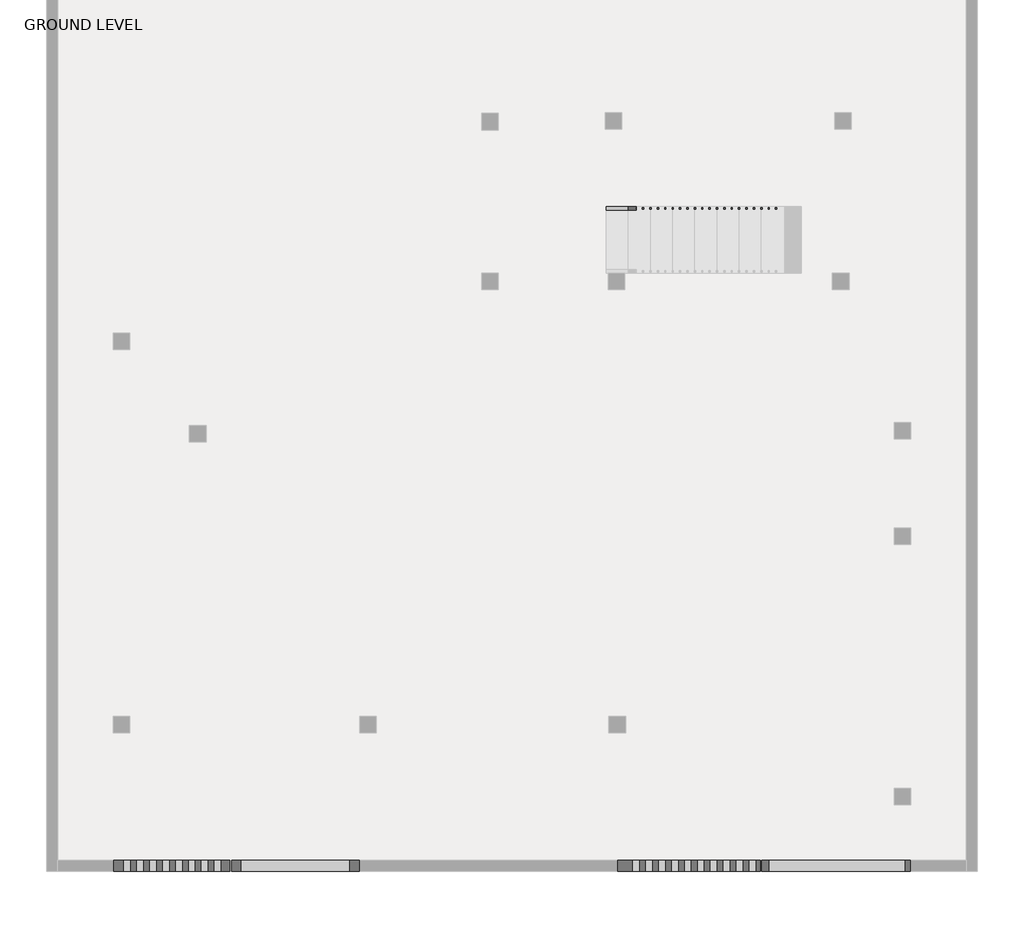
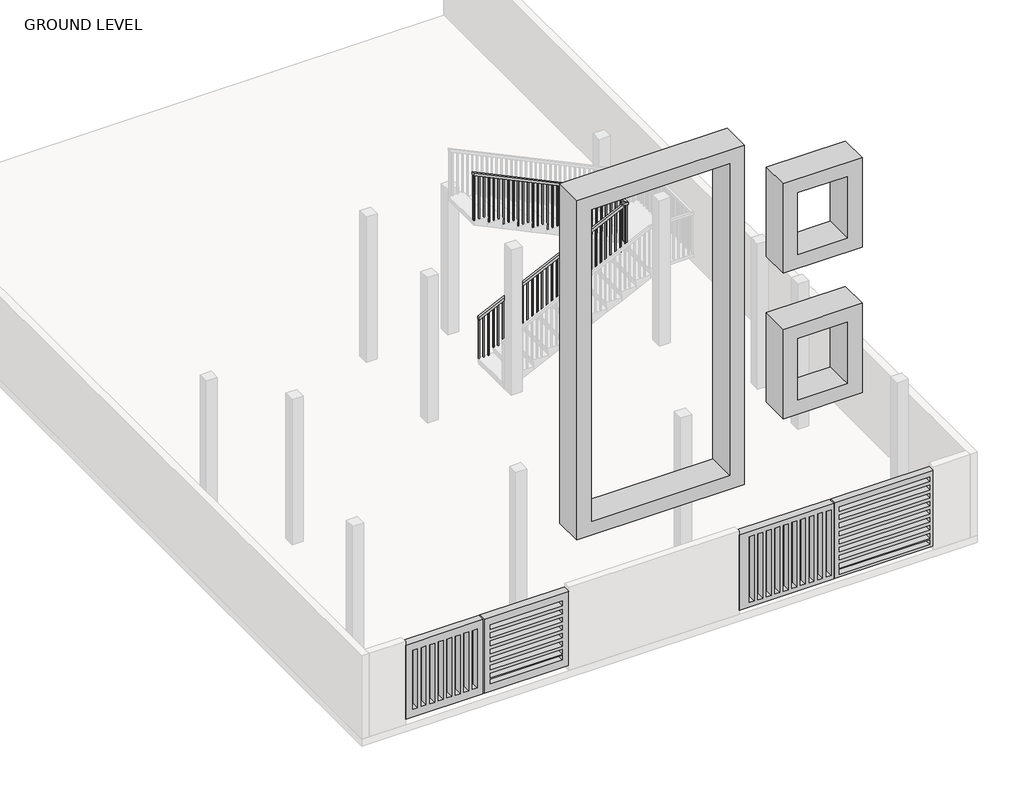
# One storey, part 3 of 3: 1 proxy, 1 railing.
"""IFC4 building model written with IfcOpenShell, lengths in millimetres."""

from ifc_helpers import new_model, si_unit, frame, origin, place, context, project, spatial, polyline, outline, extrude, faceted_brep, transform, mapped, element, save
from components import generic_models_1_generic_models_1_6b654720

model = new_model("IFC4")

# Units and contexts
model_context = context("Model", 3, world=origin())
ifc_project = project(units=[si_unit("LENGTHUNIT", "METRE", prefix="MILLI")], contexts=[model_context])

# Site, building, storey
site = spatial("IfcSite", under=ifc_project)
building = spatial("IfcBuilding", under=site)
storey = spatial("IfcBuildingStorey", under=building, Name="GROUND LEVEL", Elevation=0.0)

# Proxy
placement = place(None, origin())
generic_models_1_generic_models_1_shape = generic_models_1_generic_models_1_6b654720(model_context)
element("IfcBuildingElementProxy", 1, Name="Generic Models 1 : Generic Models 1", ObjectType="Generic Models 1 : Generic Models 1", at=placement, inside=storey, context=model_context, shape_type="MappedRepresentation", body=[
    mapped(generic_models_1_generic_models_1_shape, transform((0.0, 0.0, 0.0), x_axis=(1.0, 0.0, 0.0), y_axis=(0.0, 1.0, 0.0), z_axis=(0.0, 0.0, 1.0))),
])

# Railing
element("IfcRailing", 2, ObjectType="Handrail - Rectangular", at=placement, inside=storey, context=model_context, shape_type="SolidModel", body=[
    faceted_brep([(13.3134019, 410.1787587, 1059.8727273), (13.3134019, 410.1787587, 1003.5834559), (13.3134019, 359.3787587, 1003.5834559), (13.3134019, 359.3787587, 1059.8727273), (2985.1134019, 410.1787587, 2478.2318182), (3035.9134019, 410.1787587, 2446.1880014), (3035.9134019, 359.3787587, 2446.1880014), (2985.1134019, 359.3787587, 2478.2318182), (2985.1134019, 410.1787587, 2514.6), (3035.9134019, 410.1787587, 2463.8), (3035.9134019, 359.3787587, 2463.8), (2985.1134019, 359.3787587, 2514.6), (3061.3134019, 410.1787587, 2514.6), (3061.3134019, 410.1787587, 2463.8), (3112.1134019, 359.3787587, 2463.8), (3112.1134019, 359.3787587, 2514.6), (3061.3134019, 486.3787587, 2514.6), (3061.3134019, 537.1787587, 2463.8), (3112.1134019, 537.1787587, 2463.8), (3112.1134019, 486.3787587, 2514.6), (3061.3134019, 486.3787587, 2696.4409091), (3061.3134019, 537.1787587, 2645.6409091), (3112.1134019, 537.1787587, 2645.6409091), (3112.1134019, 486.3787587, 2696.4409091), (3061.3134019, 562.5787587, 2696.4409091), (3061.3134019, 562.5787587, 2645.6409091), (3112.1134019, 613.3787587, 2645.6409091), (3112.1134019, 613.3787587, 2696.4409091), (2985.1134019, 562.5787587, 2696.4409091), (2973.6120715, 562.5787587, 2645.6409091), (2973.6120715, 613.3787587, 2645.6409091), (2985.1134019, 613.3787587, 2696.4409091), (13.3134019, 562.5787587, 4114.8), (13.3134019, 613.3787587, 4114.8), (13.3134019, 613.3787587, 4058.5107287), (13.3134019, 562.5787587, 4058.5107287)], [[[0, 1, 2, 3]], [[1, 0, 4, 5]], [[2, 1, 5, 6]], [[3, 2, 6, 7]], [[0, 3, 7, 4]], [[5, 4, 8, 9]], [[6, 5, 9, 10]], [[7, 6, 10, 11]], [[4, 7, 11, 8]], [[9, 8, 12, 13]], [[10, 9, 13, 14]], [[11, 10, 14, 15]], [[8, 11, 15, 12]], [[13, 12, 16, 17]], [[14, 13, 17, 18]], [[15, 14, 18, 19]], [[12, 15, 19, 16]], [[17, 16, 20, 21]], [[18, 17, 21, 22]], [[19, 18, 22, 23]], [[16, 19, 23, 20]], [[21, 20, 24, 25]], [[22, 21, 25, 26]], [[23, 22, 26, 27]], [[20, 23, 27, 24]], [[25, 24, 28, 29]], [[26, 25, 29, 30]], [[27, 26, 30, 31]], [[24, 27, 31, 28]], [[32, 33, 34, 35]], [[29, 28, 32, 35]], [[30, 29, 35, 34]], [[31, 30, 34, 33]], [[28, 31, 33, 32]]]),
    extrude(outline(polyline([(4050.9340241, 29.1884019), (3054.9272727, 29.1884019), (3054.9272727, 48.2384019), (4041.8419787, 48.2384019), (4050.9340241, 29.1884019)])), frame((0.0, 578.4537587, 0.0), z_axis=(0.0, 1.0, 0.0), x_axis=(0.0, 0.0, 1.0)), (0.0, 0.0, 1.0), 19.05),
    extrude(outline(polyline([(4002.443115, 130.7884019), (3054.9272727, 130.7884019), (3054.9272727, 149.8384019), (3993.3510696, 149.8384019), (4002.443115, 130.7884019)])), frame((0.0, 578.4537587, 0.0), z_axis=(0.0, 1.0, 0.0), x_axis=(0.0, 0.0, 1.0)), (0.0, 0.0, 1.0), 19.05),
    extrude(outline(polyline([(3953.9522059, 232.3884019), (3054.9272727, 232.3884019), (3054.9272727, 251.4384019), (3944.8601605, 251.4384019), (3953.9522059, 232.3884019)])), frame((0.0, 578.4537587, 0.0), z_axis=(0.0, 1.0, 0.0), x_axis=(0.0, 0.0, 1.0)), (0.0, 0.0, 1.0), 19.05),
    extrude(outline(polyline([(3905.4612969, 333.9884019), (2909.4545455, 333.9884019), (2909.4545455, 353.0384019), (3896.3692514, 353.0384019), (3905.4612969, 333.9884019)])), frame((0.0, 578.4537587, 0.0), z_axis=(0.0, 1.0, 0.0), x_axis=(0.0, 0.0, 1.0)), (0.0, 0.0, 1.0), 19.05),
    extrude(outline(polyline([(3856.9703878, 435.5884019), (2909.4545455, 435.5884019), (2909.4545455, 454.6384019), (3847.8783423, 454.6384019), (3856.9703878, 435.5884019)])), frame((0.0, 578.4537587, 0.0), z_axis=(0.0, 1.0, 0.0), x_axis=(0.0, 0.0, 1.0)), (0.0, 0.0, 1.0), 19.05),
    extrude(outline(polyline([(3808.4794787, 537.1884019), (2909.4545455, 537.1884019), (2909.4545455, 556.2384019), (3799.3874332, 556.2384019), (3808.4794787, 537.1884019)])), frame((0.0, 578.4537587, 0.0), z_axis=(0.0, 1.0, 0.0), x_axis=(0.0, 0.0, 1.0)), (0.0, 0.0, 1.0), 19.05),
    extrude(outline(polyline([(3759.9885696, 638.7884019), (2763.9818182, 638.7884019), (2763.9818182, 657.8384019), (3750.8965241, 657.8384019), (3759.9885696, 638.7884019)])), frame((0.0, 578.4537587, 0.0), z_axis=(0.0, 1.0, 0.0), x_axis=(0.0, 0.0, 1.0)), (0.0, 0.0, 1.0), 19.05),
    extrude(outline(polyline([(3711.4976605, 740.3884019), (2763.9818182, 740.3884019), (2763.9818182, 759.4384019), (3702.405615, 759.4384019), (3711.4976605, 740.3884019)])), frame((0.0, 578.4537587, 0.0), z_axis=(0.0, 1.0, 0.0), x_axis=(0.0, 0.0, 1.0)), (0.0, 0.0, 1.0), 19.05),
    extrude(outline(polyline([(3663.0067514, 841.9884019), (2763.9818182, 841.9884019), (2763.9818182, 861.0384019), (3653.9147059, 861.0384019), (3663.0067514, 841.9884019)])), frame((0.0, 578.4537587, 0.0), z_axis=(0.0, 1.0, 0.0), x_axis=(0.0, 0.0, 1.0)), (0.0, 0.0, 1.0), 19.05),
    extrude(outline(polyline([(3614.5158423, 943.5884019), (2618.5090909, 943.5884019), (2618.5090909, 962.6384019), (3605.4237969, 962.6384019), (3614.5158423, 943.5884019)])), frame((0.0, 578.4537587, 0.0), z_axis=(0.0, 1.0, 0.0), x_axis=(0.0, 0.0, 1.0)), (0.0, 0.0, 1.0), 19.05),
    extrude(outline(polyline([(3566.0249332, 1045.1884019), (2618.5090909, 1045.1884019), (2618.5090909, 1064.2384019), (3556.9328878, 1064.2384019), (3566.0249332, 1045.1884019)])), frame((0.0, 578.4537587, 0.0), z_axis=(0.0, 1.0, 0.0), x_axis=(0.0, 0.0, 1.0)), (0.0, 0.0, 1.0), 19.05),
    extrude(outline(polyline([(3517.5340241, 1146.7884019), (2618.5090909, 1146.7884019), (2618.5090909, 1165.8384019), (3508.4419787, 1165.8384019), (3517.5340241, 1146.7884019)])), frame((0.0, 578.4537587, 0.0), z_axis=(0.0, 1.0, 0.0), x_axis=(0.0, 0.0, 1.0)), (0.0, 0.0, 1.0), 19.05),
    extrude(outline(polyline([(3469.043115, 1248.3884019), (2473.0363636, 1248.3884019), (2473.0363636, 1267.4384019), (3459.9510696, 1267.4384019), (3469.043115, 1248.3884019)])), frame((0.0, 578.4537587, 0.0), z_axis=(0.0, 1.0, 0.0), x_axis=(0.0, 0.0, 1.0)), (0.0, 0.0, 1.0), 19.05),
    extrude(outline(polyline([(3420.5522059, 1349.9884019), (2473.0363636, 1349.9884019), (2473.0363636, 1369.0384019), (3411.4601605, 1369.0384019), (3420.5522059, 1349.9884019)])), frame((0.0, 578.4537587, 0.0), z_axis=(0.0, 1.0, 0.0), x_axis=(0.0, 0.0, 1.0)), (0.0, 0.0, 1.0), 19.05),
    extrude(outline(polyline([(3372.0612969, 1451.5884019), (2473.0363636, 1451.5884019), (2473.0363636, 1470.6384019), (3362.9692514, 1470.6384019), (3372.0612969, 1451.5884019)])), frame((0.0, 578.4537587, 0.0), z_axis=(0.0, 1.0, 0.0), x_axis=(0.0, 0.0, 1.0)), (0.0, 0.0, 1.0), 19.05),
    extrude(outline(polyline([(3323.5703878, 1553.1884019), (2327.5636364, 1553.1884019), (2327.5636364, 1572.2384019), (3314.4783423, 1572.2384019), (3323.5703878, 1553.1884019)])), frame((0.0, 578.4537587, 0.0), z_axis=(0.0, 1.0, 0.0), x_axis=(0.0, 0.0, 1.0)), (0.0, 0.0, 1.0), 19.05),
    extrude(outline(polyline([(3275.0794787, 1654.7884019), (2327.5636364, 1654.7884019), (2327.5636364, 1673.8384019), (3265.9874332, 1673.8384019), (3275.0794787, 1654.7884019)])), frame((0.0, 578.4537587, 0.0), z_axis=(0.0, 1.0, 0.0), x_axis=(0.0, 0.0, 1.0)), (0.0, 0.0, 1.0), 19.05),
    extrude(outline(polyline([(3226.5885696, 1756.3884019), (2327.5636364, 1756.3884019), (2327.5636364, 1775.4384019), (3217.4965241, 1775.4384019), (3226.5885696, 1756.3884019)])), frame((0.0, 578.4537587, 0.0), z_axis=(0.0, 1.0, 0.0), x_axis=(0.0, 0.0, 1.0)), (0.0, 0.0, 1.0), 19.05),
    extrude(outline(polyline([(3178.0976605, 1857.9884019), (2182.0909091, 1857.9884019), (2182.0909091, 1877.0384019), (3169.005615, 1877.0384019), (3178.0976605, 1857.9884019)])), frame((0.0, 578.4537587, 0.0), z_axis=(0.0, 1.0, 0.0), x_axis=(0.0, 0.0, 1.0)), (0.0, 0.0, 1.0), 19.05),
    extrude(outline(polyline([(3129.6067514, 1959.5884019), (2182.0909091, 1959.5884019), (2182.0909091, 1978.6384019), (3120.5147059, 1978.6384019), (3129.6067514, 1959.5884019)])), frame((0.0, 578.4537587, 0.0), z_axis=(0.0, 1.0, 0.0), x_axis=(0.0, 0.0, 1.0)), (0.0, 0.0, 1.0), 19.05),
    extrude(outline(polyline([(3081.1158423, 2061.1884019), (2182.0909091, 2061.1884019), (2182.0909091, 2080.2384019), (3072.0237969, 2080.2384019), (3081.1158423, 2061.1884019)])), frame((0.0, 578.4537587, 0.0), z_axis=(0.0, 1.0, 0.0), x_axis=(0.0, 0.0, 1.0)), (0.0, 0.0, 1.0), 19.05),
    extrude(outline(polyline([(3032.6249332, 2162.7884019), (2036.6181818, 2162.7884019), (2036.6181818, 2181.8384019), (3023.5328878, 2181.8384019), (3032.6249332, 2162.7884019)])), frame((0.0, 578.4537587, 0.0), z_axis=(0.0, 1.0, 0.0), x_axis=(0.0, 0.0, 1.0)), (0.0, 0.0, 1.0), 19.05),
    extrude(outline(polyline([(2984.1340241, 2264.3884019), (2036.6181818, 2264.3884019), (2036.6181818, 2283.4384019), (2975.0419787, 2283.4384019), (2984.1340241, 2264.3884019)])), frame((0.0, 578.4537587, 0.0), z_axis=(0.0, 1.0, 0.0), x_axis=(0.0, 0.0, 1.0)), (0.0, 0.0, 1.0), 19.05),
    extrude(outline(polyline([(2935.643115, 2365.9884019), (2036.6181818, 2365.9884019), (2036.6181818, 2385.0384019), (2926.5510696, 2385.0384019), (2935.643115, 2365.9884019)])), frame((0.0, 578.4537587, 0.0), z_axis=(0.0, 1.0, 0.0), x_axis=(0.0, 0.0, 1.0)), (0.0, 0.0, 1.0), 19.05),
    extrude(outline(polyline([(2887.1522059, 2467.5884019), (1891.1454545, 2467.5884019), (1891.1454545, 2486.6384019), (2878.0601605, 2486.6384019), (2887.1522059, 2467.5884019)])), frame((0.0, 578.4537587, 0.0), z_axis=(0.0, 1.0, 0.0), x_axis=(0.0, 0.0, 1.0)), (0.0, 0.0, 1.0), 19.05),
    extrude(outline(polyline([(2838.6612969, 2569.1884019), (1891.1454545, 2569.1884019), (1891.1454545, 2588.2384019), (2829.5692514, 2588.2384019), (2838.6612969, 2569.1884019)])), frame((0.0, 578.4537587, 0.0), z_axis=(0.0, 1.0, 0.0), x_axis=(0.0, 0.0, 1.0)), (0.0, 0.0, 1.0), 19.05),
    extrude(outline(polyline([(2790.1703878, 2670.7884019), (1891.1454545, 2670.7884019), (1891.1454545, 2689.8384019), (2781.0783423, 2689.8384019), (2790.1703878, 2670.7884019)])), frame((0.0, 578.4537587, 0.0), z_axis=(0.0, 1.0, 0.0), x_axis=(0.0, 0.0, 1.0)), (0.0, 0.0, 1.0), 19.05),
    extrude(outline(polyline([(2741.6794787, 2772.3884019), (1745.6727273, 2772.3884019), (1745.6727273, 2791.4384019), (2732.5874332, 2791.4384019), (2741.6794787, 2772.3884019)])), frame((0.0, 578.4537587, 0.0), z_axis=(0.0, 1.0, 0.0), x_axis=(0.0, 0.0, 1.0)), (0.0, 0.0, 1.0), 19.05),
    extrude(outline(polyline([(2693.1885696, 2873.9884019), (1745.6727273, 2873.9884019), (1745.6727273, 2893.0384019), (2684.0965241, 2893.0384019), (2693.1885696, 2873.9884019)])), frame((0.0, 578.4537587, 0.0), z_axis=(0.0, 1.0, 0.0), x_axis=(0.0, 0.0, 1.0)), (0.0, 0.0, 1.0), 19.05),
    extrude(outline(polyline([(2644.6976605, 2975.5884019), (1745.6727273, 2975.5884019), (1745.6727273, 2994.6384019), (2635.605615, 2994.6384019), (2644.6976605, 2975.5884019)])), frame((0.0, 578.4537587, 0.0), z_axis=(0.0, 1.0, 0.0), x_axis=(0.0, 0.0, 1.0)), (0.0, 0.0, 1.0), 19.05),
    extrude(outline(polyline([(3077.1884019, 476.8537587), (3077.1884019, 495.9037587), (3096.2384019, 495.9037587), (3096.2384019, 476.8537587), (3077.1884019, 476.8537587)])), frame((0.0, 0.0, 1600.2), z_axis=(0.0, 0.0, 1.0), x_axis=(1.0, 0.0, 0.0)), (0.0, 0.0, 1.0), 863.6),
    extrude(outline(polyline([(3051.7884019, 394.3037587), (3070.8384019, 394.3037587), (3070.8384019, 375.2537587), (3051.7884019, 375.2537587), (3051.7884019, 394.3037587)])), frame((0.0, 0.0, 1600.2), z_axis=(0.0, 0.0, 1.0), x_axis=(1.0, 0.0, 0.0)), (0.0, 0.0, 1.0), 863.6),
    extrude(outline(polyline([(2405.2737969, 2950.1884019), (1454.7272727, 2950.1884019), (1454.7272727, 2969.2384019), (2414.3658423, 2969.2384019), (2405.2737969, 2950.1884019)])), frame((0.0, 375.2537587, 0.0), z_axis=(0.0, 1.0, 0.0), x_axis=(0.0, 0.0, 1.0)), (0.0, 0.0, 1.0), 19.05),
    extrude(outline(polyline([(2356.7828878, 2848.5884019), (1454.7272727, 2848.5884019), (1454.7272727, 2867.6384019), (2365.8749332, 2867.6384019), (2356.7828878, 2848.5884019)])), frame((0.0, 375.2537587, 0.0), z_axis=(0.0, 1.0, 0.0), x_axis=(0.0, 0.0, 1.0)), (0.0, 0.0, 1.0), 19.05),
    extrude(outline(polyline([(2308.2919787, 2746.9884019), (1454.7272727, 2746.9884019), (1454.7272727, 2766.0384019), (2317.3840241, 2766.0384019), (2308.2919787, 2746.9884019)])), frame((0.0, 375.2537587, 0.0), z_axis=(0.0, 1.0, 0.0), x_axis=(0.0, 0.0, 1.0)), (0.0, 0.0, 1.0), 19.05),
    extrude(outline(polyline([(2259.8010696, 2645.3884019), (1309.2545455, 2645.3884019), (1309.2545455, 2664.4384019), (2268.893115, 2664.4384019), (2259.8010696, 2645.3884019)])), frame((0.0, 375.2537587, 0.0), z_axis=(0.0, 1.0, 0.0), x_axis=(0.0, 0.0, 1.0)), (0.0, 0.0, 1.0), 19.05),
    extrude(outline(polyline([(2211.3101605, 2543.7884019), (1309.2545455, 2543.7884019), (1309.2545455, 2562.8384019), (2220.4022059, 2562.8384019), (2211.3101605, 2543.7884019)])), frame((0.0, 375.2537587, 0.0), z_axis=(0.0, 1.0, 0.0), x_axis=(0.0, 0.0, 1.0)), (0.0, 0.0, 1.0), 19.05),
    extrude(outline(polyline([(2162.8192514, 2442.1884019), (1309.2545455, 2442.1884019), (1309.2545455, 2461.2384019), (2171.9112969, 2461.2384019), (2162.8192514, 2442.1884019)])), frame((0.0, 375.2537587, 0.0), z_axis=(0.0, 1.0, 0.0), x_axis=(0.0, 0.0, 1.0)), (0.0, 0.0, 1.0), 19.05),
    extrude(outline(polyline([(2114.3283423, 2340.5884019), (1163.7818182, 2340.5884019), (1163.7818182, 2359.6384019), (2123.4203878, 2359.6384019), (2114.3283423, 2340.5884019)])), frame((0.0, 375.2537587, 0.0), z_axis=(0.0, 1.0, 0.0), x_axis=(0.0, 0.0, 1.0)), (0.0, 0.0, 1.0), 19.05),
    extrude(outline(polyline([(2065.8374332, 2238.9884019), (1163.7818182, 2238.9884019), (1163.7818182, 2258.0384019), (2074.9294787, 2258.0384019), (2065.8374332, 2238.9884019)])), frame((0.0, 375.2537587, 0.0), z_axis=(0.0, 1.0, 0.0), x_axis=(0.0, 0.0, 1.0)), (0.0, 0.0, 1.0), 19.05),
    extrude(outline(polyline([(2017.3465241, 2137.3884019), (1163.7818182, 2137.3884019), (1163.7818182, 2156.4384019), (2026.4385696, 2156.4384019), (2017.3465241, 2137.3884019)])), frame((0.0, 375.2537587, 0.0), z_axis=(0.0, 1.0, 0.0), x_axis=(0.0, 0.0, 1.0)), (0.0, 0.0, 1.0), 19.05),
    extrude(outline(polyline([(1968.855615, 2035.7884019), (1018.3090909, 2035.7884019), (1018.3090909, 2054.8384019), (1977.9476605, 2054.8384019), (1968.855615, 2035.7884019)])), frame((0.0, 375.2537587, 0.0), z_axis=(0.0, 1.0, 0.0), x_axis=(0.0, 0.0, 1.0)), (0.0, 0.0, 1.0), 19.05),
    extrude(outline(polyline([(1920.3647059, 1934.1884019), (1018.3090909, 1934.1884019), (1018.3090909, 1953.2384019), (1929.4567514, 1953.2384019), (1920.3647059, 1934.1884019)])), frame((0.0, 375.2537587, 0.0), z_axis=(0.0, 1.0, 0.0), x_axis=(0.0, 0.0, 1.0)), (0.0, 0.0, 1.0), 19.05),
    extrude(outline(polyline([(1871.8737969, 1832.5884019), (1018.3090909, 1832.5884019), (1018.3090909, 1851.6384019), (1880.9658423, 1851.6384019), (1871.8737969, 1832.5884019)])), frame((0.0, 375.2537587, 0.0), z_axis=(0.0, 1.0, 0.0), x_axis=(0.0, 0.0, 1.0)), (0.0, 0.0, 1.0), 19.05),
    extrude(outline(polyline([(1823.3828878, 1730.9884019), (872.8363636, 1730.9884019), (872.8363636, 1750.0384019), (1832.4749332, 1750.0384019), (1823.3828878, 1730.9884019)])), frame((0.0, 375.2537587, 0.0), z_axis=(0.0, 1.0, 0.0), x_axis=(0.0, 0.0, 1.0)), (0.0, 0.0, 1.0), 19.05),
    extrude(outline(polyline([(1774.8919787, 1629.3884019), (872.8363636, 1629.3884019), (872.8363636, 1648.4384019), (1783.9840241, 1648.4384019), (1774.8919787, 1629.3884019)])), frame((0.0, 375.2537587, 0.0), z_axis=(0.0, 1.0, 0.0), x_axis=(0.0, 0.0, 1.0)), (0.0, 0.0, 1.0), 19.05),
    extrude(outline(polyline([(1726.4010696, 1527.7884019), (872.8363636, 1527.7884019), (872.8363636, 1546.8384019), (1735.493115, 1546.8384019), (1726.4010696, 1527.7884019)])), frame((0.0, 375.2537587, 0.0), z_axis=(0.0, 1.0, 0.0), x_axis=(0.0, 0.0, 1.0)), (0.0, 0.0, 1.0), 19.05),
    extrude(outline(polyline([(1677.9101605, 1426.1884019), (727.3636364, 1426.1884019), (727.3636364, 1445.2384019), (1687.0022059, 1445.2384019), (1677.9101605, 1426.1884019)])), frame((0.0, 375.2537587, 0.0), z_axis=(0.0, 1.0, 0.0), x_axis=(0.0, 0.0, 1.0)), (0.0, 0.0, 1.0), 19.05),
    extrude(outline(polyline([(1629.4192514, 1324.5884019), (727.3636364, 1324.5884019), (727.3636364, 1343.6384019), (1638.5112969, 1343.6384019), (1629.4192514, 1324.5884019)])), frame((0.0, 375.2537587, 0.0), z_axis=(0.0, 1.0, 0.0), x_axis=(0.0, 0.0, 1.0)), (0.0, 0.0, 1.0), 19.05),
    extrude(outline(polyline([(1580.9283423, 1222.9884019), (727.3636364, 1222.9884019), (727.3636364, 1242.0384019), (1590.0203878, 1242.0384019), (1580.9283423, 1222.9884019)])), frame((0.0, 375.2537587, 0.0), z_axis=(0.0, 1.0, 0.0), x_axis=(0.0, 0.0, 1.0)), (0.0, 0.0, 1.0), 19.05),
    extrude(outline(polyline([(1532.4374332, 1121.3884019), (581.8909091, 1121.3884019), (581.8909091, 1140.4384019), (1541.5294787, 1140.4384019), (1532.4374332, 1121.3884019)])), frame((0.0, 375.2537587, 0.0), z_axis=(0.0, 1.0, 0.0), x_axis=(0.0, 0.0, 1.0)), (0.0, 0.0, 1.0), 19.05),
    extrude(outline(polyline([(1483.9465241, 1019.7884019), (581.8909091, 1019.7884019), (581.8909091, 1038.8384019), (1493.0385696, 1038.8384019), (1483.9465241, 1019.7884019)])), frame((0.0, 375.2537587, 0.0), z_axis=(0.0, 1.0, 0.0), x_axis=(0.0, 0.0, 1.0)), (0.0, 0.0, 1.0), 19.05),
    extrude(outline(polyline([(1435.455615, 918.1884019), (581.8909091, 918.1884019), (581.8909091, 937.2384019), (1444.5476605, 937.2384019), (1435.455615, 918.1884019)])), frame((0.0, 375.2537587, 0.0), z_axis=(0.0, 1.0, 0.0), x_axis=(0.0, 0.0, 1.0)), (0.0, 0.0, 1.0), 19.05),
    extrude(outline(polyline([(1386.9647059, 816.5884019), (436.4181818, 816.5884019), (436.4181818, 835.6384019), (1396.0567514, 835.6384019), (1386.9647059, 816.5884019)])), frame((0.0, 375.2537587, 0.0), z_axis=(0.0, 1.0, 0.0), x_axis=(0.0, 0.0, 1.0)), (0.0, 0.0, 1.0), 19.05),
    extrude(outline(polyline([(1338.4737969, 714.9884019), (436.4181818, 714.9884019), (436.4181818, 734.0384019), (1347.5658423, 734.0384019), (1338.4737969, 714.9884019)])), frame((0.0, 375.2537587, 0.0), z_axis=(0.0, 1.0, 0.0), x_axis=(0.0, 0.0, 1.0)), (0.0, 0.0, 1.0), 19.05),
    extrude(outline(polyline([(1289.9828878, 613.3884019), (436.4181818, 613.3884019), (436.4181818, 632.4384019), (1299.0749332, 632.4384019), (1289.9828878, 613.3884019)])), frame((0.0, 375.2537587, 0.0), z_axis=(0.0, 1.0, 0.0), x_axis=(0.0, 0.0, 1.0)), (0.0, 0.0, 1.0), 19.05),
    extrude(outline(polyline([(1241.4919787, 511.7884019), (290.9454545, 511.7884019), (290.9454545, 530.8384019), (1250.5840241, 530.8384019), (1241.4919787, 511.7884019)])), frame((0.0, 375.2537587, 0.0), z_axis=(0.0, 1.0, 0.0), x_axis=(0.0, 0.0, 1.0)), (0.0, 0.0, 1.0), 19.05),
    extrude(outline(polyline([(1193.0010696, 410.1884019), (290.9454545, 410.1884019), (290.9454545, 429.2384019), (1202.093115, 429.2384019), (1193.0010696, 410.1884019)])), frame((0.0, 375.2537587, 0.0), z_axis=(0.0, 1.0, 0.0), x_axis=(0.0, 0.0, 1.0)), (0.0, 0.0, 1.0), 19.05),
    extrude(outline(polyline([(1144.5101605, 308.5884019), (290.9454545, 308.5884019), (290.9454545, 327.6384019), (1153.6022059, 327.6384019), (1144.5101605, 308.5884019)])), frame((0.0, 375.2537587, 0.0), z_axis=(0.0, 1.0, 0.0), x_axis=(0.0, 0.0, 1.0)), (0.0, 0.0, 1.0), 19.05),
    extrude(outline(polyline([(1096.0192514, 206.9884019), (145.4727273, 206.9884019), (145.4727273, 226.0384019), (1105.1112969, 226.0384019), (1096.0192514, 206.9884019)])), frame((0.0, 375.2537587, 0.0), z_axis=(0.0, 1.0, 0.0), x_axis=(0.0, 0.0, 1.0)), (0.0, 0.0, 1.0), 19.05),
    extrude(outline(polyline([(1047.5283423, 105.3884019), (145.4727273, 105.3884019), (145.4727273, 124.4384019), (1056.6203878, 124.4384019), (1047.5283423, 105.3884019)])), frame((0.0, 375.2537587, 0.0), z_axis=(0.0, 1.0, 0.0), x_axis=(0.0, 0.0, 1.0)), (0.0, 0.0, 1.0), 19.05),
    extrude(outline(polyline([(3077.1884019, 578.4537587), (3077.1884019, 597.5037587), (3096.2384019, 597.5037587), (3096.2384019, 578.4537587), (3077.1884019, 578.4537587)])), frame((0.0, 0.0, 1600.2), z_axis=(0.0, 0.0, 1.0), x_axis=(1.0, 0.0, 0.0)), (0.0, 0.0, 1.0), 1045.4409091),
    extrude(outline(polyline([(3077.1884019, 394.3037587), (3096.2384019, 394.3037587), (3096.2384019, 375.2537587), (3077.1884019, 375.2537587), (3077.1884019, 394.3037587)])), frame((0.0, 0.0, 1600.2), z_axis=(0.0, 0.0, 1.0), x_axis=(1.0, 0.0, 0.0)), (0.0, 0.0, 1.0), 863.6),
    extrude(outline(polyline([(4058.5107287, 13.3134019), (3054.9272727, 13.3134019), (3054.9272727, 32.3634019), (4049.4186832, 32.3634019), (4058.5107287, 13.3134019)])), frame((0.0, 578.4537587, 0.0), z_axis=(0.0, 1.0, 0.0), x_axis=(0.0, 0.0, 1.0)), (0.0, 0.0, 1.0), 19.05),
    extrude(outline(polyline([(1003.5834559, 13.3134019), (145.4727273, 13.3134019), (145.4727273, 32.3634019), (1012.6755014, 32.3634019), (1003.5834559, 13.3134019)])), frame((0.0, 375.2537587, 0.0), z_axis=(0.0, 1.0, 0.0), x_axis=(0.0, 0.0, 1.0)), (0.0, 0.0, 1.0), 19.05),
])

save(model, "model.ifc")

# Revit data of these elements
# Type "Handrail - Rectangular"
#   Assembly Code = "C2010400"
#   built-in parameter 1008612 = 0.0416667 (stored number, unit not read)
#   built-in parameter 1008611 = 0.0416667 (stored number, unit not read)
#   built-in parameter 1008609 = 0.333333 (stored number, unit not read)
#   built-in parameter 1008604 = 0.166667 (stored number, unit not read)
#   built-in parameter 1008603 = 0.166667 (stored number, unit not read)
#   Railing Height = 3' - 0"
#   built-in parameter 1008630 = 2
#   built-in parameter 1008610 = 2
#   built-in parameter 1008618 = Baluster - Square : 3/4"
# Element 1 (IfcBuildingElementProxy, "Generic Models 1 : Generic Models 1")
#   Phase Created = New Construction
#   Materials on its faces: "wood", "Earth"
# Element 2 (IfcRailing, "Handrail - Rectangular")
#   Phase Created = New Construction
# Materials
#   "wood": class "Generic", colour RGB 155 131 132, transparency 0, Cost = 0
#   "Earth": class "Generic", colour RGB 97 75 62, transparency 0, Description = "Soil", Cost = 0
